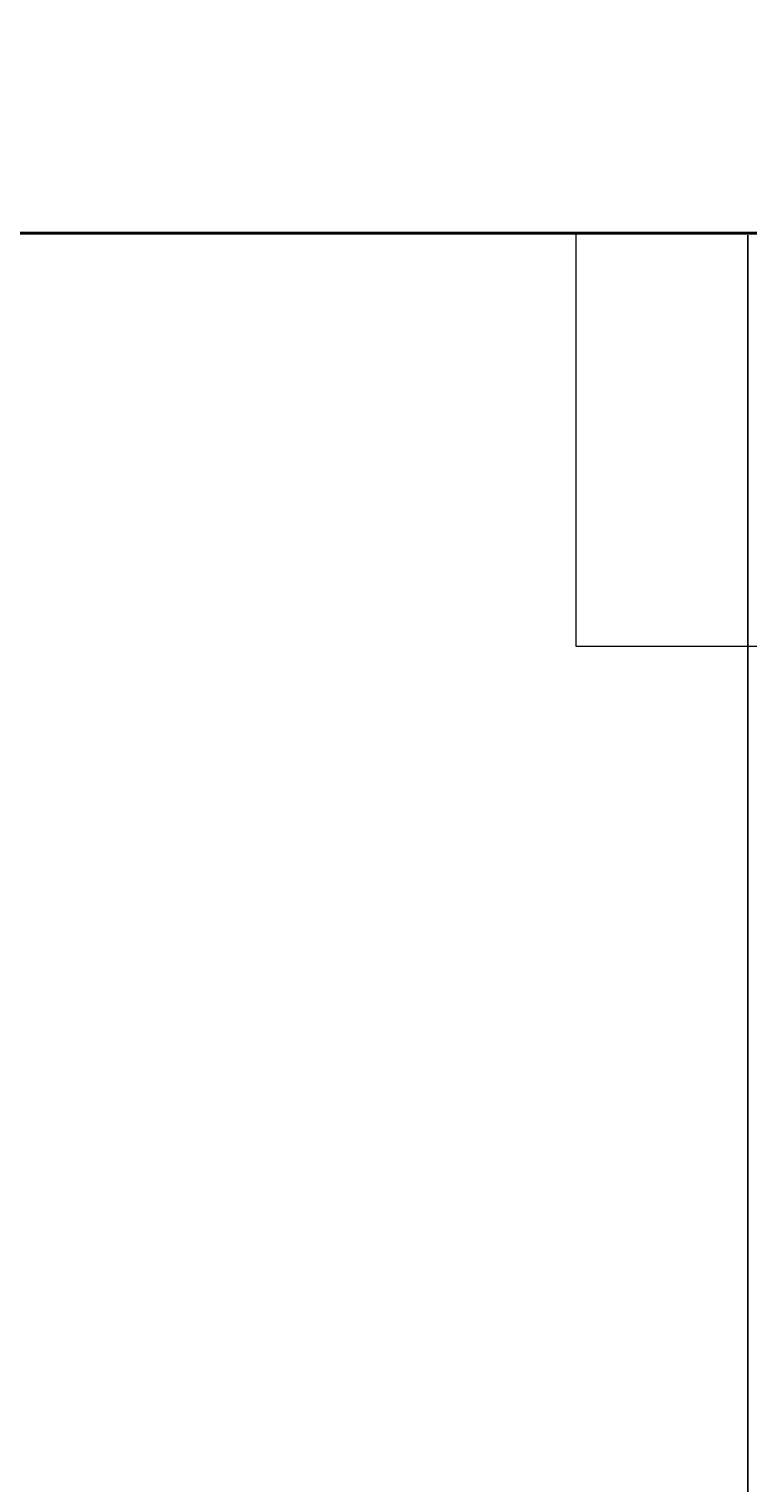
# Model space of a CAD drawing. Units: inches. Extents: x -301 to 715, y -607 to 364.
# Tile 56 of 141: x -164 to -144, y -260 to -218. Entities that reach past the tile are written whole.
import ezdxf

# ---------------------------------------------------------------- set-up
doc = ezdxf.new("R2010")
doc.units = ezdxf.units.IN
doc.header["$MEASUREMENT"] = 0
doc.linetypes.add('ACAD_ISO02W100', pattern=[15, 12, -3])
for name, color, linetype, lineweight in [('A-ANNO-DIMS', 2, 'Continuous', 18), ('A-GLAZ-OVHD', 2, 'ACAD_ISO02W100', 18), ('A-WALL', 3, 'Continuous', 40)]:
    doc.layers.add(name, color=color, linetype=linetype, lineweight=lineweight)
doc.styles.get("Standard").update_dxf_attribs({"font": 'arial.ttf'})
doc.dimstyles.get("Standard").update_dxf_attribs({"dimtxt": 0.18, "dimasz": 0.18, "dimexe": 0.18, "dimexo": 0.0625, "dimgap": 0.09, "dimtad": 0, "dimtih": 1, "dimtoh": 1, "dimdec": 1, "dimzin": 0, "dimdsep": 46, "dimlunit": 4, "dimtxsty": 'Standard', "dimcen": 0.09, "dimclrd": 3, "dimclre": 4, "dimclrt": 6, "dimadec": 0, "dimazin": 0, "dimtfac": 1, "dimtdec": 1, "dimtofl": 0, "dimtmove": 0, "dimatfit": 3, "dimfxl": 1, "dimtfill": 2, "dimtfillclr": 51, "dimtolj": 1, "dimtzin": 0, "dimarcsym": 0})

# ---------------------------------------------------------------- blocks, each defined once
blk = doc.blocks.new('WIN-SHADE-50')
at = {"ltscale": 1.5}
for p, q in [((0, 0), (0, 12)), ((50, 12), (0, 12)), ((50, 0), (50, 12)), ((5, 0), (0, 0)), ((45, 0), (50, 0))]:
    blk.add_line(p, q, dxfattribs=at)
blk = doc.blocks.new('*D146')
at = {"layer": 'A-ANNO-DIMS', "color": 4, "lineweight": -2, "transparency": 16777216}
for p, q in [((-204.603, -223.88), (-204.603, -296.865)), ((-143.603, -223.88), (-143.603, -296.865))]:
    blk.add_line(p, q, dxfattribs=at)
at = {"layer": 'A-ANNO-DIMS', "color": 3, "lineweight": -2, "transparency": 16777216}
for p, q in [((-204.423, -296.685), (-174.433, -296.685)), ((-143.783, -296.685), (-173.774, -296.685))]:
    blk.add_line(p, q, dxfattribs=at)
at = {"layer": 'A-ANNO-DIMS', "color": 3, "transparency": 16777216}
for points in [[(-204.423, -296.655), (-204.423, -296.715), (-204.603, -296.685)], [(-143.783, -296.655), (-143.783, -296.715), (-143.603, -296.685)]]:
    blk.add_solid(points, dxfattribs=at)
at = {"layer": 'Defpoints', "color": 0, "transparency": 16777216}
for p in [(-204.603, -223.818), (-143.603, -223.818), (-143.603, -296.685)]:
    blk.add_point(p, dxfattribs=at)
at = {"layer": 'A-ANNO-DIMS', "color": 6, "transparency": 16777216, "insert": (-174.103, -296.685), "char_height": 0.18, "attachment_point": 5, "bg_fill": 1, "box_fill_scale": 1.25, "bg_fill_color": 51, "bg_fill_transparency": 0}
blk.add_mtext('\\A1;5\'-1"', dxfattribs=at)
blk = doc.blocks.new('*D151')
at = {"layer": 'A-ANNO-DIMS', "color": 4, "lineweight": -2, "transparency": 16777216}
for p, q in [((-204.603, -223.755), (-204.603, 359.612)), ((-45.603, -214.755), (-45.603, 359.612))]:
    blk.add_line(p, q, dxfattribs=at)
at = {"layer": 'A-ANNO-DIMS', "color": 3, "lineweight": -2, "transparency": 16777216}
for p, q in [((-204.423, 359.432), (-125.494, 359.432)), ((-45.783, 359.432), (-124.713, 359.432))]:
    blk.add_line(p, q, dxfattribs=at)
at = {"layer": 'A-ANNO-DIMS', "color": 3, "transparency": 16777216}
for points in [[(-204.423, 359.462), (-204.423, 359.402), (-204.603, 359.432)], [(-45.783, 359.462), (-45.783, 359.402), (-45.603, 359.432)]]:
    blk.add_solid(points, dxfattribs=at)
at = {"layer": 'Defpoints', "color": 0, "transparency": 16777216}
for p in [(-45.603, 359.432), (-45.603, -214.818), (-204.603, -223.818)]:
    blk.add_point(p, dxfattribs=at)
at = {"layer": 'A-ANNO-DIMS', "color": 6, "transparency": 16777216, "insert": (-125.103, 359.432), "char_height": 0.18, "attachment_point": 5, "bg_fill": 1, "box_fill_scale": 1.25, "bg_fill_color": 51, "bg_fill_transparency": 0}
blk.add_mtext('\\A1;13\'-3"', dxfattribs=at)

msp = doc.modelspace()

# ---------------------------------------------------------------- linework, layer by layer
at = {"layer": 'A-WALL'}
msp.add_line((-204.603, -223.818), (-45.603, -223.818), dxfattribs=at)

# ---------------------------------------------------------------- block references
at = {"layer": 'A-GLAZ-OVHD', "rotation": 180}
msp.add_blockref('WIN-SHADE-50', (-98.604, -223.817), dxfattribs=at)

# ---------------------------------------------------------------- dimensions: what is measured, and where the dimension line sits
at = {"layer": 'A-ANNO-DIMS'}
for base, p2, picture, middle in [((-45.603, 359.432), (-45.603, -214.818), '*D151', (-125.103, 359.432)), ((-143.603, -296.685), (-143.603, -223.818), '*D146', (-174.103, -296.685))]:
    dim = msp.add_linear_dim(base=base, p1=(-204.603, -223.818), p2=p2, dimstyle='Standard', override={"dimdec": 1, "dimlfac": 1, "dimrnd": 0, "dimzin": 1, "dimdsep": 46, "dimlunit": 4, "dimfrac": 2}, dxfattribs=at)
    dim.commit()
    dim.dimension.update_dxf_attribs({"geometry": picture, "text_midpoint": middle})

doc.saveas('drawing.dxf')
